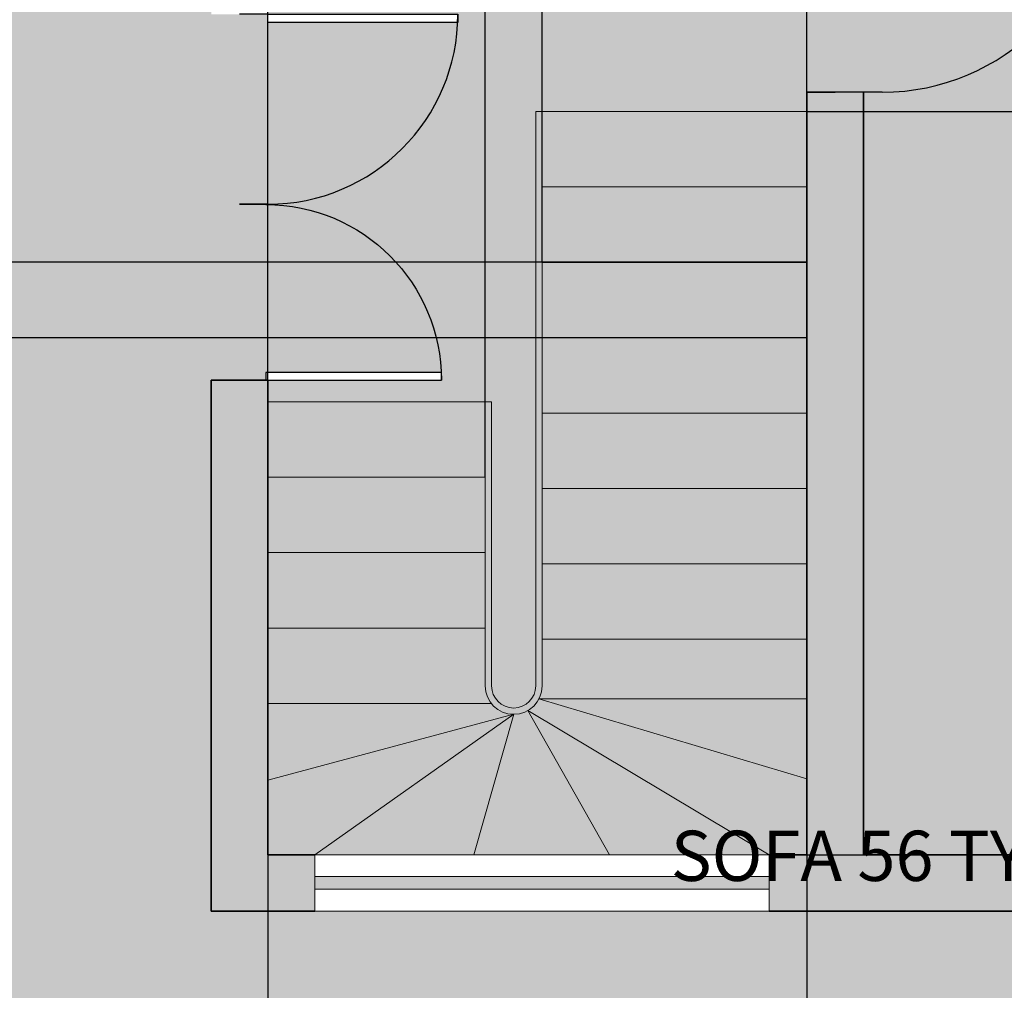
# Model space of a CAD drawing. Units: inches. Extents: x 389 to 971, y 148 to 870.
# Tile 4 of 14: x 565 to 722, y 273 to 428. Entities that reach past the tile are written whole.
import ezdxf

# ---------------------------------------------------------------- set-up
doc = ezdxf.new("R2010")
doc.units = ezdxf.units.IN
doc.header["$MEASUREMENT"] = 0
for name, color, linetype, lineweight in [('A-ANNO-DIMS', 2, 'Continuous', 18), ('A-DOOR', 4, 'Continuous', 25), ('A-FLOR-BASE-PATT', 8, 'Continuous', 13), ('A-FLOR-STRS', 7, 'Continuous', 20), ('A-GLAZ', 4, 'Continuous', 18), ('A-WALL', 7, 'Continuous', 35), ('L-GRND-BASE-PATT', 8, 'Continuous', 13)]:
    doc.layers.add(name, color=color, linetype=linetype, lineweight=lineweight)
for name, color, linetype, lineweight, true_color in [('A-FLOR-STRS-PATT', 9, 'Continuous', 13, 0xd6bdce), ('A-GLAZ-PATT', 251, 'Continuous', 13, 0x6d5f6c), ('A-WALL-PATT', 18, 'Continuous', 13, 0x000000), ('L-GRND-PATT', 39, 'Continuous', 13, 0x603913)]:
    doc.layers.add(name, color=color, linetype=linetype, lineweight=lineweight, true_color=true_color)
doc.styles.get("Standard").update_dxf_attribs({"font": 'arial.ttf'})
doc.dimstyles.get("Standard").update_dxf_attribs({"dimtxt": 8, "dimasz": 8, "dimexe": 0.18, "dimexo": 0.0625, "dimgap": 0.09, "dimtad": 0, "dimtih": 1, "dimtoh": 1, "dimdec": 0, "dimzin": 0, "dimdsep": 46, "dimlunit": 3, "dimtxsty": 'Standard', "dimcen": 0.09, "dimadec": 0, "dimazin": 0, "dimtfac": 1, "dimtdec": 0, "dimtofl": 0, "dimtmove": 0, "dimatfit": 3, "dimfxl": 1, "dimtolj": 1, "dimtzin": 0, "dimarcsym": 0})

# ---------------------------------------------------------------- blocks, each defined once
blk = doc.blocks.new('*U5')
for p, q in [((0, 0), (0, -6)), ((28, 0), (28, -6))]:
    blk.add_line(p, q)
blk.add_lwpolyline([(0, 0), (0, 28), (1.75, 28), (1.75, 0)], close=True)
blk.add_arc((0, 0), 28, 0, 90)
blk = doc.blocks.new('*U2')
for p, q in [((0, 0), (0, -6)), ((40, 0), (40, -6))]:
    blk.add_line(p, q)
blk.add_lwpolyline([(0, 0), (0, 40), (1.75, 40), (1.75, 0)], close=True)
blk.add_arc((0, 0), 40, 0, 90)
blk = doc.blocks.new('*D38')
at = {"layer": 'A-ANNO-DIMS', "color": 0, "lineweight": -2, "transparency": 16777216}
for p, q in [((746.14, 302.8), (746.14, 294.28)), ((802.17, 302.8), (802.17, 294.28)), ((746.14, 294.46), (738.14, 294.46)), ((794.17, 294.46), (754.14, 294.46))]:
    blk.add_line(p, q, dxfattribs=at)
at = {"layer": 'A-ANNO-DIMS', "color": 0, "transparency": 16777216}
for points in [[(754.14, 295.79), (754.14, 293.12), (746.14, 294.46)], [(794.17, 295.79), (794.17, 293.12), (802.17, 294.46)]]:
    blk.add_solid(points, dxfattribs=at)
at = {"layer": 'Defpoints', "color": 0, "transparency": 16777216}
for p in [(746.14, 302.86), (802.17, 302.86), (746.14, 294.46)]:
    blk.add_point(p, dxfattribs=at)
at = {"layer": 'A-ANNO-DIMS', "color": 0, "transparency": 16777216, "insert": (701.83, 294.46), "char_height": 8, "attachment_point": 5}
blk.add_mtext('\\A1;SOFA 56 TYP.', dxfattribs=at)
blk = doc.blocks.new('*D50')
at = {"layer": 'A-ANNO-DIMS', "color": 0, "lineweight": -2, "transparency": 16777216}
for p, q in [((604.39, 294.58), (604.39, 199.5)), ((690.22, 294.58), (690.22, 199.5)), ((612.39, 199.68), (633.71, 199.68)), ((682.22, 199.68), (660.89, 199.68))]:
    blk.add_line(p, q, dxfattribs=at)
at = {"layer": 'A-ANNO-DIMS', "color": 0, "transparency": 16777216}
for points in [[(612.39, 201.01), (612.39, 198.34), (604.39, 199.68)], [(682.22, 201.01), (682.22, 198.34), (690.22, 199.68)]]:
    blk.add_solid(points, dxfattribs=at)
at = {"layer": 'Defpoints', "color": 0, "transparency": 16777216}
for p in [(604.39, 294.64), (690.22, 294.64), (690.22, 199.68)]:
    blk.add_point(p, dxfattribs=at)
at = {"layer": 'A-ANNO-DIMS', "color": 0, "transparency": 16777216, "insert": (647.3, 199.68), "char_height": 8, "attachment_point": 5}
blk.add_mtext('\\A1;85.83', dxfattribs=at)
blk = doc.blocks.new('*D51')
at = {"layer": 'A-ANNO-DIMS', "color": 0, "lineweight": -2, "transparency": 16777216}
for p, q in [((596.39, 864.97), (588.39, 864.97)), ((604.39, 354.78), (604.39, 865.15)), ((639.03, 354.78), (639.03, 865.15)), ((647.03, 864.97), (655.03, 864.97))]:
    blk.add_line(p, q, dxfattribs=at)
at = {"layer": 'A-ANNO-DIMS', "color": 0, "transparency": 16777216}
for points in [[(596.39, 866.3), (596.39, 863.64), (604.39, 864.97)], [(647.03, 866.3), (647.03, 863.64), (639.03, 864.97)]]:
    blk.add_solid(points, dxfattribs=at)
at = {"layer": 'Defpoints', "color": 0, "transparency": 16777216}
for p in [(639.03, 864.97), (604.39, 354.72), (639.03, 354.72)]:
    blk.add_point(p, dxfattribs=at)
at = {"layer": 'A-ANNO-DIMS', "color": 0, "transparency": 16777216, "insert": (621.71, 864.97), "char_height": 8, "attachment_point": 5}
blk.add_mtext('\\A1;34.64', dxfattribs=at)
blk = doc.blocks.new('*D52')
at = {"layer": 'A-ANNO-DIMS', "color": 0, "lineweight": -2, "transparency": 16777216}
for p, q in [((640.06, 864.97), (632.06, 864.97)), ((648.06, 388.98), (648.06, 865.15)), ((690.22, 388.98), (690.22, 865.15)), ((698.22, 864.97), (706.22, 864.97))]:
    blk.add_line(p, q, dxfattribs=at)
at = {"layer": 'A-ANNO-DIMS', "color": 0, "transparency": 16777216}
for points in [[(640.06, 866.3), (640.06, 863.64), (648.06, 864.97)], [(698.22, 866.3), (698.22, 863.64), (690.22, 864.97)]]:
    blk.add_solid(points, dxfattribs=at)
at = {"layer": 'Defpoints', "color": 0, "transparency": 16777216}
for p in [(690.22, 864.97), (648.06, 388.92), (690.22, 388.92)]:
    blk.add_point(p, dxfattribs=at)
at = {"layer": 'A-ANNO-DIMS', "color": 0, "transparency": 16777216, "insert": (669.14, 864.97), "char_height": 8, "attachment_point": 5}
blk.add_mtext('\\A1;42.155', dxfattribs=at)
blk = doc.blocks.new('*D53')
at = {"layer": 'A-ANNO-DIMS', "color": 0, "lineweight": -2, "transparency": 16777216}
for p, q in [((397.89, 396.92), (397.89, 404.92)), ((690.15, 388.92), (397.71, 388.92)), ((690.15, 376.92), (397.71, 376.92)), ((397.89, 368.92), (397.89, 360.92))]:
    blk.add_line(p, q, dxfattribs=at)
at = {"layer": 'A-ANNO-DIMS', "color": 0, "transparency": 16777216}
for points in [[(396.56, 396.92), (399.22, 396.92), (397.89, 388.92)], [(396.56, 368.92), (399.22, 368.92), (397.89, 376.92)]]:
    blk.add_solid(points, dxfattribs=at)
at = {"layer": 'Defpoints', "color": 0, "transparency": 16777216}
for p in [(397.89, 388.92), (690.22, 388.92), (690.22, 376.92)]:
    blk.add_point(p, dxfattribs=at)
at = {"layer": 'A-ANNO-DIMS', "color": 0, "transparency": 16777216, "insert": (397.89, 382.92), "char_height": 8, "attachment_point": 5}
blk.add_mtext('\\A1;12', dxfattribs=at)
blk = doc.blocks.new('*D54')
at = {"layer": 'A-ANNO-DIMS', "color": 0, "lineweight": -2, "transparency": 16777216}
for p, q in [((690.28, 412.92), (878.72, 412.92)), ((878.54, 404.92), (878.54, 357.96)), ((878.54, 302.64), (878.54, 349.61)), ((690.28, 294.64), (878.72, 294.64))]:
    blk.add_line(p, q, dxfattribs=at)
at = {"layer": 'A-ANNO-DIMS', "color": 0, "transparency": 16777216}
for points in [[(877.21, 404.92), (879.87, 404.92), (878.54, 412.92)], [(877.21, 302.64), (879.87, 302.64), (878.54, 294.64)]]:
    blk.add_solid(points, dxfattribs=at)
at = {"layer": 'Defpoints', "color": 0, "transparency": 16777216}
for p in [(690.22, 412.92), (878.54, 412.92), (690.22, 294.64)]:
    blk.add_point(p, dxfattribs=at)
at = {"layer": 'A-ANNO-DIMS', "color": 0, "transparency": 16777216, "insert": (878.54, 353.78), "char_height": 8, "attachment_point": 5}
blk.add_mtext('\\A1;118.27', dxfattribs=at)

msp = doc.modelspace()

# ---------------------------------------------------------------- hatches: boundary and pattern name
at = {"layer": 'A-FLOR-BASE-PATT'}
h = msp.add_hatch(color=256, dxfattribs=at)
h.dxf.hatch_style = 1
h.paths.add_polyline_path([(634.6594, 428.4021), (634.6594, 427.0792), (634.6305, 427.0792, -0.40145271), (604.4225, 398.1652), (604.0817, 398.1199, -0.40145271), (632.0195, 371.3788), (632.0462, 371.3788), (632.0462, 370.1554), (604.387, 370.1554), (604.387, 366.7191), (640.0296, 366.7191), (640.0296, 321.4969, 1), (647.061, 321.4969), (647.061, 412.9189), (690.216, 412.9189), (690.216, 416.0006), (694.716, 416.0006), (702.2145, 416.0006, 0.39601219), (737.1392, 448.8066), (702.2145, 448.8066), (702.2145, 450.9936), (694.716, 450.9936), (690.216, 450.9936), (690.216, 466.6012), (708.7881, 466.6012), (708.7881, 462.1012), (784.6145, 462.1012), (784.6145, 466.6012), (794.216, 466.6012), (794.216, 591.6445), (708.5171, 591.6445), (708.5171, 596.1445), (708.5171, 602.9755, 0.39601219), (678.6314, 634.7912), (678.6314, 602.9755), (676.6391, 602.9755), (676.6391, 596.1445), (676.6391, 591.6445), (661.216, 591.6445), (661.216, 632.6445), (653.109, 632.6445), (653.109, 641.6445), (653.109, 642.1751), (651.6417, 642.1751), (651.6417, 675.6801, 0.40145271), (619.5719, 642.1751), (619.5719, 637.1445), (619.5147, 632.6445), (604.387, 632.6445), (604.387, 545.7317), (595.3894, 545.7317), (595.3894, 544.4199), (565.4338, 544.4199, 0.40145271), (595.3894, 515.7475), (599.887, 515.7475), (604.387, 515.7271), (604.387, 428.4021)])
h.paths.add_polyline_path([(721.8003, 493.9292), (725.0899, 493.9292), (725.0899, 493.075), (751.4065, 493.075), (751.4065, 493.9292), (754.6961, 493.9292), (754.6961, 479.6744, -0.26666697), (721.8003, 479.6744)], flags=16)
h.paths.add_polyline_path([(720.6421, 516.0583), (720.6421, 545.0393), (753.5806, 545.0393), (753.5806, 516.0583)], flags=16)
h.paths.add_polyline_path([(722.6421, 518.0583), (722.6421, 543.0393), (751.5806, 543.0393), (751.5806, 518.0583)], flags=0)
h.paths.add_polyline_path([(763.7396, 488.5801), (763.7822, 488.1156), (764.1436, 488.1761)], flags=16)
h.paths.add_polyline_path([(777.9011, 479.7417), (778.0475, 480.1886), (777.4745, 480.275)], flags=16)
h.paths.add_polyline_path([(762.3329, 503.5919), (762.3329, 507.1718), (763.2624, 507.1718), (763.2624, 550.1306), (762.3329, 550.1306), (762.3329, 553.7105), (777.8458, 553.7105, -0.19047621), (777.8458, 503.5919)], flags=16)
h.paths.add_polyline_path([(721.6097, 567.2898), (721.6097, 581.7362, -0.26666697), (754.9475, 581.7362), (754.9475, 567.2898), (751.6137, 567.2898), (751.6137, 568.1555), (724.9435, 568.1555), (724.9435, 567.2898)], flags=16)
h.paths.add_polyline_path([(774.6347, 521.4914), (774.6347, 535.811), (778.6837, 535.811, -0.04962821), (778.6837, 521.4914)], flags=0)
h.paths.add_polyline_path([(764.6624, 576.8996), (764.7454, 576.4742), (765.0717, 576.4903)], flags=16)
h.paths.add_polyline_path([(777.2772, 570.3652), (777.4444, 570.8756), (776.7899, 570.9743)], flags=16)
h.paths.add_polyline_path([(644.2892, 516.9956), (685.2491, 516.9956), (685.2491, 535.7223), (644.2892, 535.7223)], flags=24)
h = msp.add_hatch(color=256, dxfattribs=at)
h.dxf.hatch_style = 1
h.paths.add_polyline_path([(699.216, 294.6445), (733.8057, 294.6445), (810.0514, 294.6445), (839.216, 294.6445), (839.216, 457.6012), (784.6145, 457.6012), (784.6145, 462.1012), (708.7881, 462.1012), (708.7881, 457.6012), (699.216, 457.6012), (699.216, 450.9936), (702.2145, 450.9936), (737.2076, 450.9936), (737.2076, 448.8066), (737.1392, 448.8066, -0.39601219), (702.2145, 416.0006), (699.216, 416.0006)])
h.paths.add_polyline_path([(755.1859, 373.9163), (788.1244, 373.9163), (788.1244, 344.9352), (755.1859, 344.9352)], flags=16)
h.paths.add_polyline_path([(757.1859, 371.9163), (786.1244, 371.9163), (786.1244, 346.9352), (757.1859, 346.9352)], flags=0)
h.paths.add_polyline_path([(746.1376, 327.3223), (750.14, 327.3223), (750.14, 326.2831), (798.1694, 326.2831), (798.1694, 327.3223), (802.1718, 327.3223), (802.1718, 309.9784, -0.19047621), (746.1376, 309.9784)], flags=16)
h.paths.add_polyline_path([(782.1596, 313.5685), (782.1596, 309.0415, -0.04962821), (766.1498, 309.0415), (766.1498, 313.5685)], flags=0)
h.paths.add_polyline_path([(804.6838, 390.5197), (803.6446, 390.5197), (803.6446, 394.5221), (820.9885, 394.5221, -0.19047621), (820.9885, 338.4879), (803.6446, 338.4879), (803.6446, 342.4903), (804.6838, 342.4903)], flags=16)
h.paths.add_polyline_path([(817.3984, 358.5001), (817.3984, 374.5099), (821.9254, 374.5099, -0.04962821), (821.9254, 358.5001)], flags=0)
h.paths.add_polyline_path([(806.8707, 326.6963), (806.4254, 327.1416), (806.4724, 326.6297)], flags=16)
h.paths.add_polyline_path([(822.0328, 317.4008), (822.1942, 317.8933), (821.5626, 317.9885)], flags=16)
h.paths.add_polyline_path([(808.1446, 418.9737), (808.2247, 418.5632), (808.5395, 418.5787)], flags=16)
h.paths.add_polyline_path([(820.3159, 412.669), (820.4772, 413.1615), (819.8457, 413.2568)], flags=16)
h.paths.add_polyline_path([(750.6082, 393.6667), (791.5681, 393.6667), (791.5681, 412.3933), (750.6082, 412.3933)], flags=24)
at = {"layer": 'A-FLOR-STRS-PATT'}
h = msp.add_hatch(color=256, dxfattribs=at)
h.dxf.hatch_style = 1
h.paths.add_polyline_path([(647.061, 321.4969, -1), (640.0296, 321.4969), (640.0296, 366.7191), (639.0296, 366.7191), (639.0296, 321.4969, 1), (648.061, 321.4969), (648.061, 412.9189), (647.061, 412.9189)])
h = msp.add_hatch(color=256, dxfattribs=at)
h.dxf.hatch_style = 1
h.paths.add_polyline_path([(690.216, 400.9189), (690.216, 412.9189), (648.061, 412.9189), (648.061, 400.9189)])
h = msp.add_hatch(color=256, dxfattribs=at)
h.dxf.hatch_style = 1
h.paths.add_polyline_path([(690.216, 388.9189), (690.216, 400.9189), (648.061, 400.9189), (648.061, 388.9189)])
h = msp.add_hatch(color=256, dxfattribs=at)
h.dxf.hatch_style = 1
h.paths.add_polyline_path([(648.061, 388.9189), (648.061, 376.9189), (690.216, 376.9189), (690.216, 388.9189)])
h = msp.add_hatch(color=256, dxfattribs=at)
h.dxf.hatch_style = 1
h.paths.add_polyline_path([(690.216, 364.9189), (690.216, 376.9189), (648.061, 376.9189), (648.061, 364.9189)])
h = msp.add_hatch(color=256, dxfattribs=at)
h.dxf.hatch_style = 1
h.paths.add_polyline_path([(639.0296, 354.7191), (639.0296, 366.7191), (604.387, 366.7191), (604.387, 354.7191)])
h = msp.add_hatch(color=256, dxfattribs=at)
h.dxf.hatch_style = 1
h.paths.add_polyline_path([(648.061, 364.9189), (648.061, 352.9189), (690.216, 352.9189), (690.216, 364.9189)])
h = msp.add_hatch(color=256, dxfattribs=at)
h.dxf.hatch_style = 1
h.paths.add_polyline_path([(639.0296, 342.7191), (639.0296, 354.7191), (604.387, 354.7191), (604.387, 342.7191)])
h = msp.add_hatch(color=256, dxfattribs=at)
h.dxf.hatch_style = 1
h.paths.add_polyline_path([(690.216, 340.9189), (690.216, 352.9189), (648.061, 352.9189), (648.061, 340.9189)])
h = msp.add_hatch(color=256, dxfattribs=at)
h.dxf.hatch_style = 1
h.paths.add_polyline_path([(639.0296, 330.7191), (639.0296, 342.7191), (604.387, 342.7191), (604.387, 330.7191)])
h = msp.add_hatch(color=256, dxfattribs=at)
h.dxf.hatch_style = 1
h.paths.add_polyline_path([(690.216, 328.9189), (690.216, 340.9189), (648.061, 340.9189), (648.061, 328.9189)])
h = msp.add_hatch(color=256, dxfattribs=at)
h.dxf.hatch_style = 1
h.paths.add_polyline_path([(639.985, 318.7191, -0.16717054), (639.0296, 321.4969), (639.0296, 330.7191), (604.387, 330.7191), (604.387, 318.7191)])
h = msp.add_hatch(color=256, dxfattribs=at)
h.dxf.hatch_style = 1
h.paths.add_polyline_path([(690.216, 319.4616), (690.216, 328.9189), (648.061, 328.9189), (648.061, 321.4969, -0.1174302), (647.5763, 319.4616)])
h = msp.add_hatch(color=256, dxfattribs=at)
h.dxf.hatch_style = 1
h.paths.add_polyline_path([(643.5453, 316.9812, -0.2310445), (639.985, 318.7191), (604.387, 318.7191), (604.387, 306.5071)])
h = msp.add_hatch(color=256, dxfattribs=at)
h.dxf.hatch_style = 1
h.paths.add_polyline_path([(684.2434, 294.6445), (690.216, 294.6445), (690.216, 306.6966), (647.5763, 319.4616, -0.14615064), (645.7997, 317.5842)])
h = msp.add_hatch(color=256, dxfattribs=at)
h.dxf.hatch_style = 1
h.paths.add_polyline_path([(690.216, 306.6966), (690.216, 319.4616), (647.5763, 319.4616)])
h = msp.add_hatch(color=256, dxfattribs=at)
h.dxf.hatch_style = 1
h.paths.add_polyline_path([(643.5453, 316.9812), (604.387, 306.5071), (604.387, 294.6445), (611.8787, 294.6445)])
h = msp.add_hatch(color=256, dxfattribs=at)
h.dxf.hatch_style = 1
h.paths.add_polyline_path([(643.5453, 316.9812), (611.8787, 294.6445), (637.1816, 294.6445)])
h = msp.add_hatch(color=256, dxfattribs=at)
h.dxf.hatch_style = 1
h.paths.add_polyline_path([(658.7908, 294.6445), (645.7997, 317.5842, -0.13143008), (643.5453, 316.9812), (637.1816, 294.6445)])
h = msp.add_hatch(color=256, dxfattribs=at)
h.dxf.hatch_style = 1
h.paths.add_polyline_path([(645.7997, 317.5842), (658.7908, 294.6445), (684.2434, 294.6445)])
at = {"layer": 'A-GLAZ-PATT'}
h = msp.add_hatch(color=256, dxfattribs=at)
h.dxf.hatch_style = 1
h.paths.add_polyline_path([(684.2434, 289.1445), (684.2434, 291.1445), (611.8787, 291.1445), (611.8787, 289.1445)])
h = msp.add_hatch(color=256, dxfattribs=at)
h.dxf.hatch_style = 1
h.paths.add_polyline_path([(611.8787, 291.1445), (611.8787, 289.1445), (684.2434, 289.1445), (684.2434, 291.1445)])
at = {"layer": 'A-WALL-PATT'}
h = msp.add_hatch(color=256, dxfattribs=at)
h.dxf.hatch_style = 1
h.paths.add_polyline_path([(690.216, 294.6445), (684.2434, 294.6445), (684.2434, 285.6445), (733.8057, 285.6445), (733.8057, 294.6445), (699.216, 294.6445), (699.216, 416.0006), (694.716, 416.0006), (690.216, 416.0006)])
h = msp.add_hatch(color=256, dxfattribs=at)
h.dxf.hatch_style = 1
h.paths.add_polyline_path([(690.216, 294.6445), (684.2434, 294.6445), (684.2434, 285.6445), (733.8057, 285.6445), (733.8057, 294.6445), (699.216, 294.6445), (699.216, 400.9189), (690.216, 400.9189)])
h = msp.add_hatch(color=256, dxfattribs=at)
h.dxf.hatch_style = 1
h.paths.add_polyline_path([(604.387, 370.1554), (604.0817, 370.1554), (599.887, 370.1554), (595.387, 370.1554), (595.387, 285.6445), (604.387, 285.6445), (611.8787, 285.6445), (611.8787, 294.6445), (604.387, 294.6445)])
at = {"layer": 'L-GRND-BASE-PATT'}
h = msp.add_hatch(color=256, dxfattribs=at)
h.dxf.hatch_style = 1
edge = h.paths.add_edge_path(flags=16)
edge.add_ellipse((8782.0026, 354.2473), major_axis=(-8296.9493, 0), ratio=0.84230387, start_angle=-0.09022909, end_angle=0.38386678, ccw=False)
edge.add_ellipse((485.0533, 368.2895), major_axis=(-1.1591, 0), ratio=0.84230387, start_angle=0, end_angle=90, ccw=False)
edge.add_line((483.8943, 368.2895), (483.8943, 387.6039))
edge.add_ellipse((485.0533, 387.2466), major_axis=(1.1591, 0), ratio=0.84230387, start_angle=90, end_angle=180, ccw=False)
edge.add_line((485.0533, 388.2229), (485.5047, 388.2229))
edge.add_ellipse((898.8202, 372.4897), major_axis=(413.7374, 0), ratio=0.84230387, start_angle=176.349572, end_angle=177.82005, ccw=False)
edge.add_ellipse((535.9119, 196.3855), major_axis=(-245.3972, 0), ratio=0.84230387, start_angle=-77.874034, end_angle=-76.219471, ccw=False)
edge.add_ellipse((535.9119, 201.7547), major_axis=(239.1274, 0), ratio=0.84230387, start_angle=100.209539, end_angle=102.444627, ccw=False)
edge.add_ellipse((473.3139, 564.9222), major_axis=(196.5637, 0), ratio=0.84230387, start_angle=-80.743434, end_angle=-77.445067)
edge.add_line((509.5535, 402.1941), (514.3535, 404.8483))
edge.add_line((514.3535, 404.8483), (514.3535, 404.7972))
edge.add_ellipse((514.3535, 404.2644), major_axis=(0.5795, 0), ratio=0.84230387, start_angle=52.06687, end_angle=90, ccw=False)
edge.add_line((514.6716, 404.6725), (519.1535, 402.1941))
edge.add_ellipse((555.3932, 564.9222), major_axis=(-196.5637, 0), ratio=0.84230387, start_angle=77.445067, end_angle=80.743434)
edge.add_ellipse((492.7951, 201.7547), major_axis=(239.1274, 0), ratio=0.84230387, start_angle=77.555373, end_angle=79.790461, ccw=False)
edge.add_ellipse((492.7951, 196.3855), major_axis=(245.3972, 0), ratio=0.84230387, start_angle=76.219471, end_angle=77.874034, ccw=False)
edge.add_ellipse((129.8868, 372.4897), major_axis=(-413.7374, 0), ratio=0.84230387, start_angle=182.17995, end_angle=183.650428, ccw=False)
edge.add_line((543.2023, 388.2229), (544.0779, 388.2229))
edge.add_ellipse((543.6537, 387.2466), major_axis=(-1.1591, 0), ratio=0.84230387, start_angle=180, end_angle=270, ccw=False)
edge.add_line((544.8128, 387.2466), (544.8128, 367.9322))
edge.add_ellipse((543.6537, 368.2895), major_axis=(1.1591, 0), ratio=0.84230387, start_angle=270, end_angle=360, ccw=False)
edge.add_ellipse((-7753.2956, 354.2473), major_axis=(-8296.9493, 0), ratio=0.84230387, start_angle=179.61613322, end_angle=180.09022909, ccw=False)
edge.add_line((543.3912, 298.6608), (544.0779, 298.6608))
edge.add_ellipse((543.6537, 297.6845), major_axis=(1.1591, 0), ratio=0.84230387, start_angle=0, end_angle=90, ccw=False)
edge.add_line((544.8128, 297.6845), (544.8128, 278.3701))
edge.add_ellipse((543.6537, 278.7275), major_axis=(-1.1591, 0), ratio=0.84230387, start_angle=90, end_angle=180, ccw=False)
edge.add_line((543.6537, 277.7512), (543.1566, 277.7512))
edge.add_ellipse((-7753.2956, 354.2473), major_axis=(-8296.9493, 0), ratio=0.84230387, start_angle=179.3813568, end_angle=179.47172853, ccw=False)
edge.add_ellipse((542.4236, 263.2763), major_axis=(-1.7386, 0), ratio=0.84230387, start_angle=179.371763, end_angle=248.464757, ccw=False)
edge.add_ellipse((-7753.8751, 354.2473), major_axis=(-8298.7403, 0), ratio=0.842303866, start_angle=179.35344592, end_angle=179.3717628, ccw=False)
edge.add_ellipse((540.0116, 260.6509), major_axis=(-4.1092, 0), ratio=0.84230387, start_angle=90, end_angle=179.353446, ccw=False)
edge.add_line((540.0116, 257.1897), (488.6954, 257.1897))
edge.add_ellipse((488.6954, 260.6509), major_axis=(4.1092, 0), ratio=0.84230387, start_angle=180.646554, end_angle=270, ccw=False)
edge.add_ellipse((8782.5821, 354.2473), major_axis=(-8298.7403, 0), ratio=0.842303872, start_angle=0.62823723, end_angle=0.64655411, ccw=False)
edge.add_ellipse((486.2834, 263.2763), major_axis=(-1.7386, 0), ratio=0.84230387, start_angle=-68.464756, end_angle=0.628237, ccw=False)
edge.add_ellipse((8782.0026, 354.2473), major_axis=(-8296.9493, 0), ratio=0.84230387, start_angle=0.52827147, end_angle=0.6465541, ccw=False)
edge.add_line((485.5504, 277.7512), (484.6291, 277.7512))
edge.add_ellipse((485.0533, 278.7275), major_axis=(-1.1591, 0), ratio=0.84230387, start_angle=0, end_angle=90, ccw=False)
edge.add_line((483.8943, 278.7275), (483.8943, 298.0418))
edge.add_ellipse((485.0533, 297.6845), major_axis=(1.1591, 0), ratio=0.84230387, start_angle=90, end_angle=180, ccw=False)
edge = h.paths.add_edge_path(flags=0)
edge.add_ellipse((8782.0026, 354.2473), major_axis=(-8295.7902, 0), ratio=0.84230387, start_angle=0.05559431, end_angle=0.37776419, ccw=False)
edge.add_line((486.2179, 346.1978), (489.3905, 335.8384))
edge.add_ellipse((3386.0114, 329.7263), major_axis=(-2896.63, 0), ratio=0.84230387, start_angle=-0.1208974, end_angle=0.3640763)
edge.add_line((489.4638, 311.3204), (486.4666, 299.5521))
edge = h.paths.add_edge_path(flags=0)
edge.add_ellipse((514.3535, 391.3731), major_axis=(-115.1513, 0), ratio=0.84230387, start_angle=76.401865, end_angle=103.598135)
edge.add_line((537.3428, 296.3333), (537.3428, 281.5897))
edge.add_ellipse((514.3535, 376.6295), major_axis=(-115.1513, 0), ratio=0.84230387, start_angle=76.401865, end_angle=103.598135, ccw=False)
edge.add_line((491.3643, 281.5897), (491.3643, 296.3333))
edge = h.paths.add_edge_path(flags=0)
edge.add_line((491.3643, 337.0752), (489.653, 349.9016))
edge.add_ellipse((510.1338, 298.7862), major_axis=(64.0481, 0), ratio=0.84230387, start_angle=94.277421, end_angle=111.834954, ccw=False)
edge.add_line((506.1068, 352.6274), (522.6002, 352.6274))
edge.add_ellipse((518.5732, 298.7862), major_axis=(64.0481, 0), ratio=0.84230387, start_angle=68.165046, end_angle=85.722579, ccw=False)
edge.add_line((539.0541, 349.9016), (537.3428, 337.0752))
edge.add_ellipse((516.5462, 287.5825), major_axis=(62.3305, 0), ratio=0.84230387, start_angle=67.208085, end_angle=85.12993)
edge.add_line((521.008, 339.949), (507.699, 339.949))
edge.add_ellipse((512.1609, 287.5825), major_axis=(62.3305, 0), ratio=0.84230387, start_angle=94.87007, end_angle=112.791915)
edge = h.paths.add_edge_path(flags=0)
edge.add_ellipse((493.6824, 273.9439), major_axis=(-2.3182, 0), ratio=0.84230387, start_angle=-90, end_angle=0, ccw=False)
edge.add_line((493.6824, 275.8965), (535.3743, 275.8965))
edge.add_ellipse((535.0246, 273.9439), major_axis=(2.3182, 0), ratio=0.84230387, start_angle=0, end_angle=90, ccw=False)
edge.add_line((537.3428, 273.9439), (537.3428, 258.6983))
edge.add_line((537.3428, 258.6983), (540.5912, 258.6983))
edge.add_ellipse((540.5912, 260.6509), major_axis=(-2.3182, 0), ratio=0.84230387, start_angle=90, end_angle=179.353446)
edge.add_line((540.5912, 258.6983), (487.7691, 258.6983))
edge.add_ellipse((488.1158, 260.6509), major_axis=(2.3182, 0), ratio=0.84230387, start_angle=180.646554, end_angle=270)
edge.add_line((488.1158, 258.6983), (491.3643, 258.6983))
edge.add_line((491.3643, 258.6983), (491.3643, 274.2384))
h.paths.add_polyline_path([(746.1376, 327.3223), (750.14, 327.3223), (750.14, 326.2831), (798.1694, 326.2831), (798.1694, 327.3223), (802.1718, 327.3223), (802.1718, 309.9784, -0.19047621), (746.1376, 309.9784)], flags=16)
h.paths.add_polyline_path([(782.1596, 313.5685), (782.1596, 309.0415, -0.04962821), (766.1498, 309.0415), (766.1498, 313.5685)], flags=0)
h.paths.add_polyline_path([(755.1859, 344.9352), (755.1859, 373.9163), (788.1244, 373.9163), (788.1244, 344.9352)], flags=16)
h.paths.add_polyline_path([(757.1859, 346.9352), (757.1859, 371.9163), (786.1244, 371.9163), (786.1244, 346.9352)], flags=0)
h.paths.add_polyline_path([(803.6446, 338.4879), (803.6446, 342.4903), (804.6838, 342.4903), (804.6838, 390.5197), (803.6446, 390.5197), (803.6446, 394.5221), (820.9885, 394.5221, -0.19047621), (820.9885, 338.4879)], flags=16)
h.paths.add_polyline_path([(806.8707, 326.6963), (806.4254, 327.1416), (806.4724, 326.6297)], flags=16)
h.paths.add_polyline_path([(822.0328, 317.4008), (822.1942, 317.8933), (821.5626, 317.9885)], flags=16)
h.paths.add_polyline_path([(817.3984, 358.5001), (817.3984, 374.5099), (821.9254, 374.5099, -0.04962821), (821.9254, 358.5001)], flags=0)
h.paths.add_polyline_path([(808.1446, 418.9737), (808.2247, 418.5632), (808.5395, 418.5787)], flags=16)
h.paths.add_polyline_path([(820.3159, 412.669), (820.4772, 413.1615), (819.8457, 413.2568)], flags=16)
h.paths.add_polyline_path([(466.3155, 235.5246), (517.3807, 235.5246), (517.3807, 244.4269), (466.3155, 244.4269)], flags=24)
h.paths.add_polyline_path([(739.8737, 256.2), (815.404, 256.2), (815.404, 265.3454), (739.8737, 265.3454)], flags=24)
h.paths.add_polyline_path([(750.6082, 393.6667), (791.5681, 393.6667), (791.5681, 412.3933), (750.6082, 412.3933)], flags=24)
h.paths.add_polyline_path([(438.9631, 410.0619), (484.6204, 410.0619), (484.6204, 429.1217), (438.9631, 429.1217)], flags=24)
edge = h.paths.add_edge_path()
edge.add_line((839.216, 285.6445), (611.8787, 285.6445))
edge.add_line((611.8787, 285.6445), (604.387, 285.6445))
edge.add_line((604.387, 285.6445), (595.387, 285.6445))
edge.add_line((595.387, 285.6445), (595.387, 370.1554))
edge.add_line((595.387, 370.1554), (604.0817, 370.1554))
edge.add_line((604.0817, 370.1554), (604.0817, 371.3788))
edge.add_line((604.0817, 371.3788), (632.0195, 371.3788))
edge.add_arc((604.0817, 370.1554), 27.9645, 2.507491, 90)
edge.add_line((604.0817, 398.1199), (599.887, 398.1652))
edge.add_line((599.887, 398.1652), (604.4225, 398.1652))
edge.add_arc((604.4225, 428.4021), 30.2369, 270, 357.492509)
edge.add_line((634.6305, 427.0792), (604.4225, 427.0792))
edge.add_line((604.4225, 427.0792), (604.4225, 428.4021))
edge.add_line((604.4225, 428.4021), (599.887, 428.4021))
edge.add_line((599.887, 428.4021), (595.387, 428.4021))
edge.add_line((595.387, 428.4021), (595.387, 434.6445))
edge.add_line((595.387, 434.6445), (585.0791, 434.6445))
edge.add_line((585.0791, 434.6445), (540.3922, 434.6445))
edge.add_line((540.3922, 434.6445), (526.7125, 434.6445))
edge.add_line((526.7125, 434.6445), (488.4095, 434.6445))
edge.add_line((488.4095, 434.6445), (432.216, 434.6445))
edge.add_line((432.216, 434.6445), (432.216, 243.6445))
edge.add_line((432.216, 243.6445), (437.216, 243.6445))
edge.add_line((437.216, 243.6445), (437.216, 234.6445))
edge.add_line((437.216, 234.6445), (581.216, 234.6445))
edge.add_line((581.216, 234.6445), (581.216, 238.6445))
edge.add_line((581.216, 238.6445), (581.216, 243.6445))
edge.add_line((581.216, 243.6445), (590.216, 243.6445))
edge.add_line((590.216, 243.6445), (590.216, 238.6445))
edge.add_line((590.216, 238.6445), (839.216, 238.6445))
edge.add_line((839.216, 238.6445), (839.216, 285.6445))
at = {"layer": 'L-GRND-PATT'}
h = msp.add_hatch(dxfattribs=at)
h.set_pattern_fill('EARTH', color=256, angle=45)
h.set_pattern_definition([(45, (0, 0), (0, 8.980256), [6.35, -6.35]), (45, (-1.684, 1.684), (0, 8.980256), [6.35, -6.35]), (45, (-3.3676, 3.3676), (0, 8.980256), [6.35, -6.35]), (135, (-3.3676, 4.49), (-8.980256, 0), [6.35, -6.35]), (135, (-1.684, 6.174), (-8.980256, 0), [6.35, -6.35]), (135, (0, 7.858), (-8.980256, 0), [6.35, -6.35])])
h.paths.add_polyline_path([(432.216, 243.6445), (437.216, 243.6445), (437.216, 234.6445), (581.216, 234.6445), (581.216, 238.6445), (581.216, 243.6445), (590.216, 243.6445), (590.216, 238.6445), (839.216, 238.6445), (839.216, 285.6445), (810.0514, 285.6445), (733.8057, 285.6445), (684.2434, 285.6445), (611.8787, 285.6445), (604.387, 285.6445), (595.387, 285.6445), (595.387, 370.1554), (604.0817, 370.1554), (604.0817, 371.3788), (632.0195, 371.3788, 0.40145271), (604.0817, 398.1199), (599.887, 398.1652), (604.4225, 398.1652, 0.40145271), (634.6305, 427.0792), (604.4225, 427.0792), (604.4225, 428.4021), (599.887, 428.4021), (595.387, 428.4021), (595.387, 434.6445), (585.0791, 434.6445), (540.3922, 434.6445), (526.7125, 434.6445), (488.4095, 434.6445), (432.216, 434.6445)])
edge = h.paths.add_edge_path(flags=16)
edge.add_line((483.8943, 278.7275), (483.8943, 298.2564))
edge.add_ellipse((485.0533, 297.6845), major_axis=(1.1591, 0), ratio=0.84230387, start_angle=90, end_angle=180, ccw=False)
edge.add_ellipse((8782.0026, 354.2473), major_axis=(-8296.9493, 0), ratio=0.84230387, start_angle=-0.09022909, end_angle=0.38386678, ccw=False)
edge.add_ellipse((485.0533, 368.2895), major_axis=(-1.1591, 0), ratio=0.84230387, start_angle=0, end_angle=90, ccw=False)
edge.add_line((483.8943, 368.2895), (483.8943, 387.8185))
edge.add_ellipse((485.0533, 387.2466), major_axis=(1.1591, 0), ratio=0.84230387, start_angle=90, end_angle=180, ccw=False)
edge.add_ellipse((898.8202, 372.4897), major_axis=(413.7374, 0), ratio=0.84230387, start_angle=176.349572, end_angle=177.82005, ccw=False)
edge.add_ellipse((535.9119, 196.3855), major_axis=(-245.3972, 0), ratio=0.84230387, start_angle=-77.874034, end_angle=-76.219471, ccw=False)
edge.add_ellipse((535.9119, 201.7547), major_axis=(239.1274, 0), ratio=0.84230387, start_angle=100.209539, end_angle=102.444627, ccw=False)
edge.add_ellipse((473.3139, 564.9222), major_axis=(196.5637, 0), ratio=0.84230387, start_angle=-80.743434, end_angle=-77.445067)
edge.add_line((509.5535, 402.1941), (514.3535, 404.8483))
edge.add_line((514.3535, 404.8483), (519.1535, 402.1941))
edge.add_ellipse((555.3932, 564.9222), major_axis=(-196.5637, 0), ratio=0.84230387, start_angle=77.445067, end_angle=80.743434)
edge.add_ellipse((492.7951, 201.7547), major_axis=(239.1274, 0), ratio=0.84230387, start_angle=77.555373, end_angle=79.790461, ccw=False)
edge.add_ellipse((492.7951, 196.3855), major_axis=(245.3972, 0), ratio=0.84230387, start_angle=76.219471, end_angle=77.874034, ccw=False)
edge.add_ellipse((129.8868, 372.4897), major_axis=(-413.7374, 0), ratio=0.84230387, start_angle=182.17995, end_angle=183.650428, ccw=False)
edge.add_line((543.2023, 388.2229), (544.3327, 388.2229))
edge.add_ellipse((543.6537, 387.2466), major_axis=(-1.1591, 0), ratio=0.84230387, start_angle=180, end_angle=270, ccw=False)
edge.add_line((544.8128, 387.2466), (544.8128, 367.7176))
edge.add_ellipse((543.6537, 368.2895), major_axis=(1.1591, 0), ratio=0.84230387, start_angle=270, end_angle=360, ccw=False)
edge.add_ellipse((-7753.2956, 354.2473), major_axis=(-8296.9493, 0), ratio=0.84230387, start_angle=179.61613322, end_angle=180.09022909, ccw=False)
edge.add_ellipse((543.6537, 297.6845), major_axis=(1.1591, 0), ratio=0.84230387, start_angle=0, end_angle=90, ccw=False)
edge.add_line((544.8128, 297.6845), (544.8128, 278.1556))
edge.add_ellipse((543.6537, 278.7275), major_axis=(-1.1591, 0), ratio=0.84230387, start_angle=90, end_angle=180, ccw=False)
edge.add_ellipse((-7753.2956, 354.2473), major_axis=(-8296.9493, 0), ratio=0.84230387, start_angle=179.3813568, end_angle=179.47172853, ccw=False)
edge.add_ellipse((542.4236, 263.2763), major_axis=(-1.7386, 0), ratio=0.84230387, start_angle=179.371763, end_angle=248.464757, ccw=False)
edge.add_ellipse((-7753.8751, 354.2473), major_axis=(-8298.7403, 0), ratio=0.842303866, start_angle=179.35344592, end_angle=179.3717628, ccw=False)
edge.add_ellipse((540.0116, 260.6509), major_axis=(-4.1092, 0), ratio=0.84230387, start_angle=90, end_angle=179.353446, ccw=False)
edge.add_line((540.0116, 257.1897), (488.0808, 257.1897))
edge.add_ellipse((488.6954, 260.6509), major_axis=(4.1092, 0), ratio=0.84230387, start_angle=180.646554, end_angle=270, ccw=False)
edge.add_ellipse((8782.5821, 354.2473), major_axis=(-8298.7403, 0), ratio=0.842303872, start_angle=0.62823723, end_angle=0.64655411, ccw=False)
edge.add_ellipse((486.2834, 263.2763), major_axis=(-1.7386, 0), ratio=0.84230387, start_angle=-68.464756, end_angle=0.628237, ccw=False)
edge.add_ellipse((8782.0026, 354.2473), major_axis=(-8296.9493, 0), ratio=0.84230387, start_angle=0.52827147, end_angle=0.6465541, ccw=False)
edge.add_line((485.5504, 277.7512), (484.3744, 277.7512))
edge.add_ellipse((485.0533, 278.7275), major_axis=(-1.1591, 0), ratio=0.84230387, start_angle=0, end_angle=90, ccw=False)
edge = h.paths.add_edge_path(flags=0)
edge.add_ellipse((488.1158, 260.6509), major_axis=(2.3182, 0), ratio=0.84230387, start_angle=180.646554, end_angle=270)
edge.add_line((488.1158, 258.6983), (491.3643, 258.6983))
edge.add_line((491.3643, 258.6983), (491.3643, 274.4686))
edge.add_ellipse((493.6824, 273.9439), major_axis=(-2.3182, 0), ratio=0.84230387, start_angle=-90, end_angle=0, ccw=False)
edge.add_line((493.6824, 275.8965), (535.6476, 275.8965))
edge.add_ellipse((535.0246, 273.9439), major_axis=(2.3182, 0), ratio=0.84230387, start_angle=0, end_angle=90, ccw=False)
edge.add_line((537.3428, 273.9439), (537.3428, 258.6983))
edge.add_line((537.3428, 258.6983), (541.2086, 258.6983))
edge.add_ellipse((540.5912, 260.6509), major_axis=(-2.3182, 0), ratio=0.84230387, start_angle=90, end_angle=179.353446, ccw=False)
edge.add_line((540.5912, 258.6983), (487.4984, 258.6983))
edge = h.paths.add_edge_path(flags=0)
edge.add_line((491.3643, 281.5897), (491.3643, 296.3333))
edge.add_ellipse((514.3535, 391.3731), major_axis=(-115.1513, 0), ratio=0.84230387, start_angle=76.401865, end_angle=103.598135)
edge.add_line((537.3428, 296.3333), (537.3428, 281.5897))
edge.add_ellipse((514.3535, 376.6295), major_axis=(-115.1513, 0), ratio=0.84230387, start_angle=76.401865, end_angle=103.598135, ccw=False)
edge = h.paths.add_edge_path(flags=0)
edge.add_ellipse((8782.0026, 354.2473), major_axis=(-8295.7902, 0), ratio=0.84230387, start_angle=0.05559431, end_angle=0.37776419, ccw=False)
edge.add_line((486.2179, 346.1978), (489.3905, 335.8384))
edge.add_ellipse((3386.0114, 329.7263), major_axis=(-2896.63, 0), ratio=0.84230387, start_angle=-0.1208974, end_angle=0.3640763)
edge.add_line((489.4638, 311.3204), (486.4666, 299.5521))
edge = h.paths.add_edge_path(flags=0)
edge.add_line((491.3643, 337.0752), (489.653, 349.9016))
edge.add_ellipse((510.1338, 298.7862), major_axis=(64.0481, 0), ratio=0.84230387, start_angle=94.277421, end_angle=111.834954, ccw=False)
edge.add_line((506.1068, 352.6274), (522.6002, 352.6274))
edge.add_ellipse((518.5732, 298.7862), major_axis=(64.0481, 0), ratio=0.84230387, start_angle=68.165046, end_angle=85.722579, ccw=False)
edge.add_line((539.0541, 349.9016), (537.3428, 337.0752))
edge.add_ellipse((516.5462, 287.5825), major_axis=(62.3305, 0), ratio=0.84230387, start_angle=67.208085, end_angle=85.12993)
edge.add_line((521.008, 339.949), (507.699, 339.949))
edge.add_ellipse((512.1609, 287.5825), major_axis=(62.3305, 0), ratio=0.84230387, start_angle=94.87007, end_angle=112.791915)
h.paths.add_polyline_path([(466.3155, 235.5246), (517.3807, 235.5246), (517.3807, 244.4269), (466.3155, 244.4269)], flags=24)
h.paths.add_polyline_path([(739.8737, 256.2), (815.404, 256.2), (815.404, 265.3454), (739.8737, 265.3454)], flags=24)
h.paths.add_polyline_path([(438.9631, 410.0619), (484.6204, 410.0619), (484.6204, 429.1217), (438.9631, 429.1217)], flags=24)

# ---------------------------------------------------------------- linework, layer by layer
at = {"layer": 'A-FLOR-STRS'}
for p, q in [((647.061, 412.9189), (647.061, 321.4969)), ((690.216, 412.9189), (647.061, 412.9189)), ((648.061, 412.9189), (648.061, 321.4969)), ((690.216, 400.9189), (648.061, 400.9189)), ((690.216, 388.9189), (648.061, 388.9189)), ((690.216, 376.9189), (648.061, 376.9189)), ((604.387, 366.7191), (640.0296, 366.7191)), ((639.0296, 366.7191), (639.0296, 321.4969)), ((640.0296, 366.7191), (640.0296, 321.4969)), ((690.216, 364.9189), (648.061, 364.9189)), ((604.387, 354.7191), (639.0296, 354.7191)), ((690.216, 352.9189), (648.061, 352.9189)), ((604.387, 342.7191), (639.0296, 342.7191)), ((690.216, 340.9189), (648.061, 340.9189)), ((604.387, 330.7191), (639.0296, 330.7191)), ((690.216, 328.9189), (648.061, 328.9189)), ((604.387, 318.7191), (639.985, 318.7191)), ((690.216, 319.4616), (647.5763, 319.4616)), ((647.5763, 319.4616), (690.216, 306.6966)), ((604.387, 306.5071), (643.5453, 316.9812)), ((611.8787, 294.6445), (643.5453, 316.9812)), ((637.1816, 294.6445), (643.5453, 316.9812)), ((658.7908, 294.6445), (645.7997, 317.5842)), ((645.7997, 317.5842), (684.2434, 294.6445))]:
    msp.add_line(p, q, dxfattribs=at)
for radius in [4.5157, 3.5157]:
    msp.add_arc((643.5453, 321.4969), radius, 180, 0, dxfattribs=at)
at = {"layer": 'A-GLAZ'}
for p, q in [((611.8787, 294.6445), (611.8787, 285.6445)), ((611.8787, 294.6445), (684.2434, 294.6445)), ((684.2434, 294.6445), (684.2434, 285.6445)), ((611.8787, 291.1445), (684.2434, 291.1445)), ((611.8787, 289.1445), (684.2434, 289.1445)), ((611.8787, 285.6445), (684.2434, 285.6445))]:
    msp.add_line(p, q, dxfattribs=at)
at = {"layer": 'A-WALL'}
for p, q in [((690.216, 294.6445), (690.216, 416.0006)), ((694.716, 416.0006), (690.216, 416.0006)), ((699.216, 294.6445), (699.216, 416.0006)), ((595.387, 370.1554), (604.387, 370.1554)), ((595.387, 370.1554), (595.387, 285.6445)), ((604.387, 370.1554), (604.387, 294.6445)), ((611.8787, 294.6445), (604.387, 294.6445)), ((690.216, 294.6445), (684.2434, 294.6445)), ((733.8057, 294.6445), (699.216, 294.6445)), ((604.387, 285.6445), (595.387, 285.6445)), ((611.8787, 285.6445), (604.387, 285.6445)), ((733.8057, 285.6445), (684.2434, 285.6445))]:
    msp.add_line(p, q, dxfattribs=at)

# ---------------------------------------------------------------- block references
at = {"layer": 'A-DOOR', "rotation": 270}
for name, p, xscale, yscale, zscale in [('*U5', (702.2145, 450.9936), 1.249752530320971, 1.249752530320971, 1.249752530320971), ('*U2', (604.4225, 428.4021), 0.755921805587303, 0.755921805587303, 0.755921805587303), ('*U2', (604.0817, 370.1554), -0.6991135396968661, 0.6991135396968661, 0.6991135396968661)]:
    msp.add_blockref(name, p, dxfattribs=dict(at, xscale=xscale, yscale=yscale, zscale=zscale))

# ---------------------------------------------------------------- dimensions: what is measured, and where the dimension line sits
at = {"layer": 'A-ANNO-DIMS'}
for base, p1, p2, override, picture, middle in [((639.0296, 864.9695), (604.387, 354.7191), (639.0296, 354.7191), {"dimdec": 2, "dimlfac": 1, "dimrnd": 0, "dimzin": 0, "dimdsep": 46, "dimlunit": 2}, '*D51', (621.7083, 864.9695)), ((690.216, 864.9695), (648.061, 388.9189), (690.216, 388.9189), {"dimdec": 3, "dimlfac": 1, "dimrnd": 0, "dimzin": 0, "dimdsep": 46, "dimlunit": 2}, '*D52', (669.1385, 864.9695)), ((690.216, 199.6753), (604.387, 294.6445), (690.216, 294.6445), {"dimdec": 2, "dimlfac": 1, "dimrnd": 0, "dimzin": 0, "dimdsep": 46, "dimlunit": 2}, '*D50', (647.3015, 199.6753))]:
    dim = msp.add_linear_dim(base=base, p1=p1, p2=p2, dimstyle='Standard', override=override, dxfattribs=at)
    dim.commit()
    dim.dimension.update_dxf_attribs({"geometry": picture, "text_midpoint": middle})
for base, p1, p2, override, picture, middle in [((878.541, 412.9189), (690.216, 294.6445), (690.216, 412.9189), {"dimdec": 2, "dimlfac": 1, "dimrnd": 0, "dimzin": 0, "dimdsep": 46, "dimlunit": 2}, '*D54', (878.541, 353.7817)), ((397.891, 388.9189), (690.216, 376.9189), (690.216, 388.9189), {"dimdec": 0, "dimlfac": 1, "dimrnd": 0, "dimzin": 0, "dimdsep": 46, "dimlunit": 2}, '*D53', (397.891, 382.9189))]:
    dim = msp.add_linear_dim(base=base, p1=p1, p2=p2, angle=90, dimstyle='Standard', override=override, dxfattribs=at)
    dim.commit()
    dim.dimension.update_dxf_attribs({"geometry": picture, "text_midpoint": middle})
dim = msp.add_linear_dim(base=(746.1376, 294.4578), p1=(802.1718, 302.8629), p2=(746.1376, 302.8629), angle=180, text='SOFA <> TYP.', dimstyle='Standard', override={"dimdec": 0, "dimlfac": 1, "dimrnd": 0, "dimzin": 0, "dimdsep": 46, "dimlunit": 2}, dxfattribs=at)
dim.commit()
dim.dimension.update_dxf_attribs({"geometry": '*D38', "text_midpoint": (701.8293, 294.4578)})

doc.saveas('drawing.dxf')
